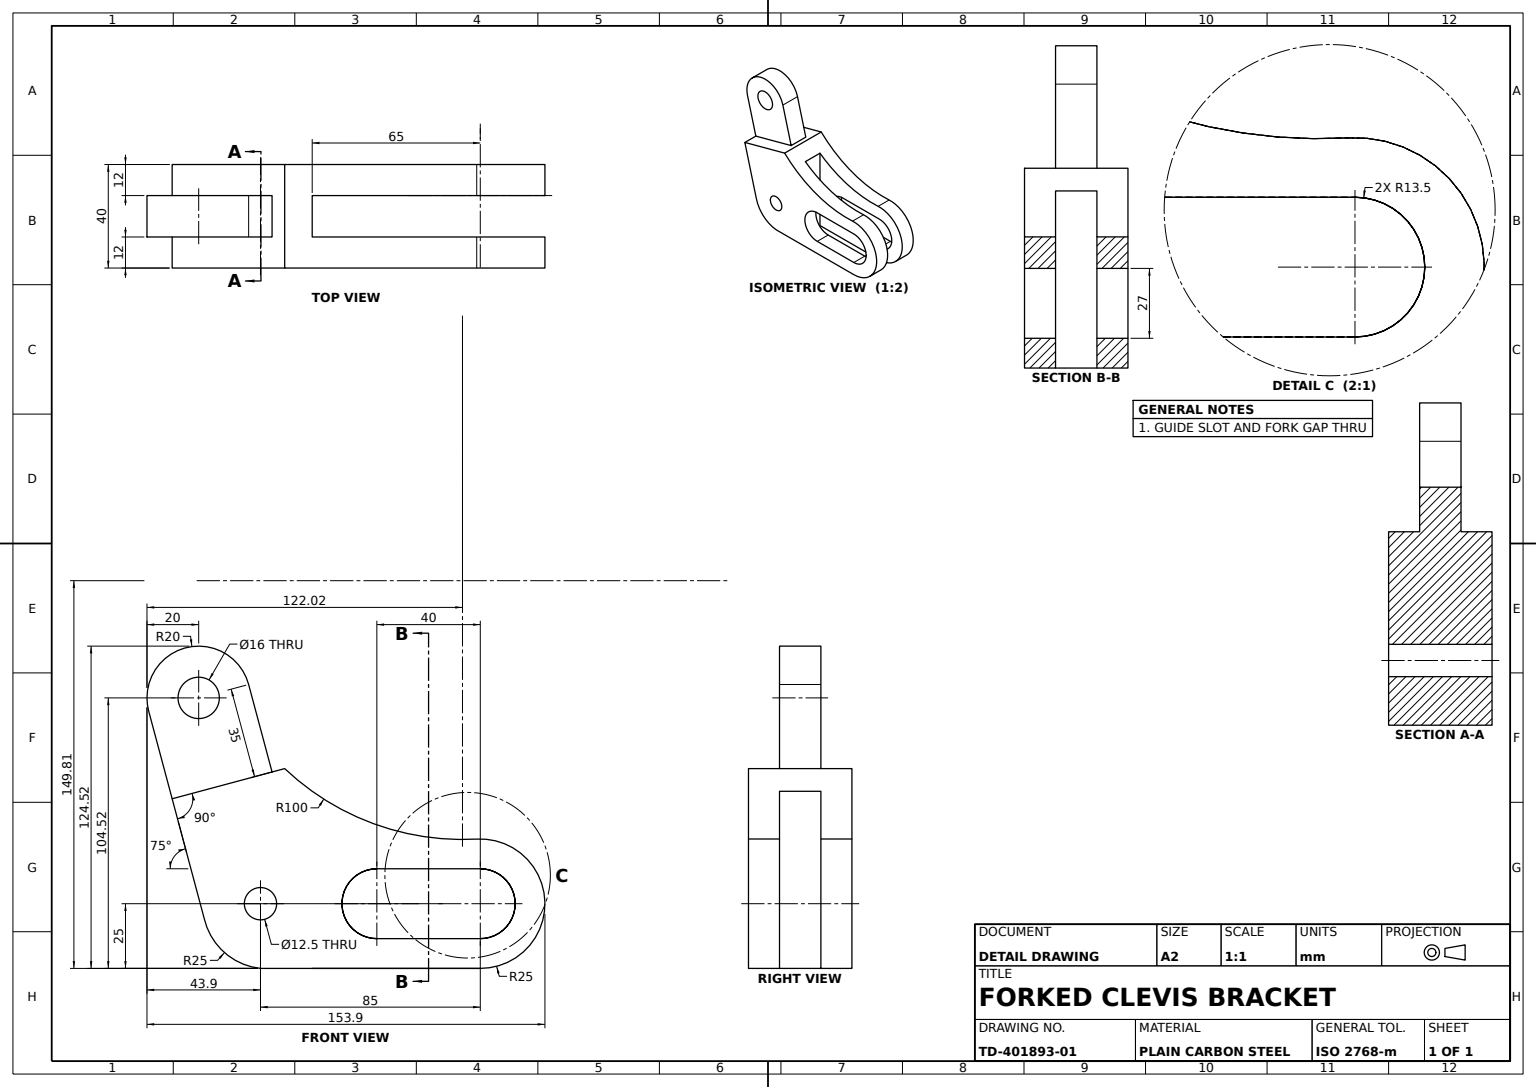
SolidWorks part; units mm, degrees
material "Plain Carbon Steel"
ref_plane "Front Plane" through (0, 0, 0) normal (0, 0, 1) x (1, 0, 0)
ref_plane "Top Plane" through (0, 0, 0) normal (0, 1, 0) x (1, 0, 0)
ref_plane "Right Plane" through (0, 0, 0) normal (1, 0, 0) x (0, 0, -1)
sketch "Base Plate Profile" plane through (0, 0, 0) normal (0, 0, 1) x (1, 0, 0)
  line L1 (0, -25) -> (-85, -25)
  line L2 (0, 0) -> (-85, 0) construction
  line L8 (-106.7333, -5.8234) -> (-119.1566, 40.541)
  line L9 (-85, 0) -> (-85, 15) construction
  line L10 (-85, 0) -> (-97.4233, 46.3644) construction
  line L11 (-119.1566, 40.541) -> (-75.6404, 52.2012)
  arc A0 (0, -25) -> (-1.3762, 24.9621) centre (0, 0) ccw
  circle A5 centre (-85, 0) radius 6.25
  arc A6 (-85, -25) -> (-106.7333, -5.8234) centre (-82.3887, -0.1368) cw
  arc A7 (-1.3762, 24.9621) -> (-75.6404, 52.2012) centre (-6.8808, 124.8105) cw
  dimension "D1" = 50
  dimension "D4" = 12.5
  dimension "D9" = 25
  dimension "D8" = 22.5
  dimension "D3" = 85
  dimension "D10" = 147.2422
  dimension "D7" = 100
  dimension "D2" = 85
  dimension "D5" = 48
  dimension "D6" = 15
extrude "Base Plate" add sketch "Base Plate Profile" along normal mid plane 40
sketch "Guide Slot Profile" plane through (0, 0, 20) normal (0, 0, 1) x (1, 0, 0)
  line L0 (0, 0) -> (-40, 0) construction
  line L1 (-40, 13.5) -> (0, 13.5)
  line L2 (-40, -13.5) -> (0, -13.5)
  arc A0 (0, -13.5) -> (0, 13.5) centre (0, 0) ccw
  arc A1 (-40, 13.5) -> (-40, -13.5) centre (-40, 0) ccw
  dimension "D1" = 27
  dimension "D2" = 40
extrude "Guide Slot" cut sketch "Guide Slot Profile" against normal through all
sketch "Fork Gap Profile" plane through (0, 0, 0) normal (0, 0, 1) x (1, 0, 0)
  line L0 (-65, 43.4338) -> (-65, -25)
  line L3 (-75.6404, 52.2012) -> (-119.1566, 40.541)
  line L4 (-119.1566, 40.541) -> (-106.7333, -5.8234)
  line L5 (-85, -25) -> (0, -25)
  line L8 (-65, -25) -> (0, -25)
  arc A3 (0, -25) -> (-1.3762, 24.9621) centre (0, 0) ccw
  arc A4 (-75.6404, 52.2012) -> (-1.3762, 24.9621) centre (-6.8808, 124.8105) ccw
  arc A5 (-106.7333, -5.8234) -> (-85, -25) centre (-82.3887, -0.1368) ccw
  arc A6 (0, -25) -> (-1.3762, 24.9621) centre (0, 0) ccw
  arc A7 (-65, 43.4338) -> (-1.3762, 24.9621) centre (-6.8808, 124.8105) ccw
  dimension "D2" = 65
  dimension "D1" = 0
extrude "Fork Gap 16mm" cut sketch "Fork Gap Profile" against normal mid plane 16
sketch "Pivot Lug Profile" plane through (0, 0, 0) normal (0, 0, 1) x (1, 0, 0)
  line L0 (-119.1566, 40.541) -> (-128.2153, 74.3484)
  line L1 (-89.5783, 84.7012) -> (-80.5196, 50.8938)
  line L2 (-80.5196, 50.8938) -> (-119.1566, 40.541)
  line L3 (-75.6404, 52.2012) -> (-119.1566, 40.541) construction
  arc A0 (-128.2153, 74.3484) -> (-89.5783, 84.7012) centre (-108.8968, 79.5248) cw
  dimension "D2" = 20
  dimension "D1" = 35
  dimension "D3" = 35
  dimension "D4" = 40
extrude "Pivot Lug" add sketch "Pivot Lug Profile" along normal mid plane 16
sketch "Pivot Hole Profile" plane through (0, 0, 8) normal (0, 0, 1) x (1, 0, 0)
  circle A0 centre (-108.8968, 79.5248) radius 8
  dimension "D1" = 16
extrude "Pivot Hole Ø16" cut sketch "Pivot Hole Profile" against normal mid plane 160
